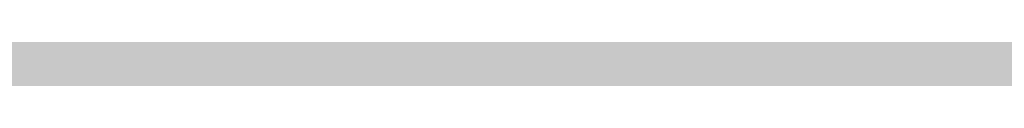
# Model space of a CAD drawing. Units: millimetres. Extents: x 0 to 2267, y 0 to 1823.
# Tile 222 of 256: x 1841.442 to 1842.748, y 1127.423 to 1127.462. Entities that reach past the tile are written whole.
import ezdxf

# ---------------------------------------------------------------- set-up
doc = ezdxf.new("R2010")
doc.units = ezdxf.units.MM
doc.header["$MEASUREMENT"] = 0
doc.layers.add('M-HATC', color=252, linetype='Continuous', lineweight=18)

msp = doc.modelspace()

# ---------------------------------------------------------------- hatches: boundary and pattern name
at = {"layer": 'M-HATC'}
h = msp.add_hatch(color=256, dxfattribs=at)
h.dxf.hatch_style = 1
h.paths.add_polyline_path([(2055.771, 1603.062), (1381.0868, 1603.062), (1381.0868, 1598.062), (2055.771, 1598.062)])
h.paths.add_polyline_path([(2055.771, 1598.062), (1381.0868, 1598.062), (1381.0868, 1593.062), (2055.771, 1593.062)])
h.paths.add_polyline_path([(2051.3074, 1536.7609), (1385.5504, 1536.7609), (1385.5504, 1526.7609), (1387.5504, 1526.7609), (1388.5366, 1525.0528), (1385.3319, 1521.2335), (1385.3319, 1521.2226), (2050.2542, 1522.7491), (2048.3212, 1525.0528), (2049.3074, 1526.7609), (2051.3074, 1526.7609)])
edge = h.paths.add_edge_path()
edge.add_arc((1847.5345, 1379.1492), 135, 222.603061, 222.890851, ccw=False)
edge.add_line((1748.1663, 1287.7656), (1683.0921, 1287.7656))
edge.add_arc((1583.7239, 1379.1492), 135, 317.109149, 317.396939, ccw=False)
edge.add_arc((1678.9686, 1290.6707), 5, 222.8909, 317.1091, ccw=False)
edge.add_arc((1774.2133, 1379.1492), 135, 222.603061, 222.890851, ccw=False)
edge.add_line((1674.8451, 1287.7656), (1609.7709, 1287.7656))
edge.add_arc((1510.4027, 1379.1492), 135, 317.109149, 317.396939, ccw=False)
edge.add_arc((1605.6474, 1290.6707), 5, 222.8909, 317.1091, ccw=False)
edge.add_arc((1700.8921, 1379.1492), 135, 222.603061, 222.890851, ccw=False)
edge.add_line((1601.5239, 1287.7656), (1536.4497, 1287.7656))
edge.add_arc((1437.0815, 1379.1492), 135, 317.109149, 317.396939, ccw=False)
edge.add_arc((1532.3262, 1290.6707), 5, 222.8909, 317.1091, ccw=False)
edge.add_arc((1627.5709, 1379.1492), 135, 222.603061, 222.890851, ccw=False)
edge.add_line((1528.2027, 1287.7656), (1505.9289, 1287.7656))
edge.add_spline(control_points=[(1505.9289, 1287.7656), (1504.2622, 1287.7656), (1504.2622, 1282.7656), (1505.9289, 1282.7656)], knot_values=[0, 0, 0, 0, 5, 5, 5, 5], degree=3, periodic=0)
edge.add_line((1505.9289, 1282.7656), (1930.9289, 1282.7656))
edge.add_spline(control_points=[(1930.9289, 1282.7656), (1932.5956, 1282.7656), (1932.5956, 1287.7656), (1930.9289, 1287.7656)], knot_values=[0, 0, 0, 0, 5, 5, 5, 5], degree=3, periodic=0)
edge.add_line((1930.9289, 1287.7656), (1903.0557, 1287.7656))
edge.add_arc((1803.6875, 1379.1492), 135, 317.109149, 317.396939, ccw=False)
edge.add_arc((1898.9322, 1290.6707), 5, 222.8909, 317.1091, ccw=False)
edge.add_arc((1994.1769, 1379.1492), 135, 222.603061, 222.890851, ccw=False)
edge.add_line((1894.8087, 1287.7656), (1829.7345, 1287.7656))
edge.add_arc((1730.3663, 1379.1492), 135, 317.109149, 317.396939, ccw=False)
edge.add_arc((1825.611, 1290.6707), 5, 222.8909, 317.1091, ccw=False)
edge.add_arc((1920.8557, 1379.1492), 135, 222.603061, 222.890851, ccw=False)
edge.add_line((1821.4875, 1287.7656), (1756.4133, 1287.7656))
edge.add_arc((1657.0451, 1379.1492), 135, 317.109149, 317.396939, ccw=False)
edge.add_arc((1752.2898, 1290.6707), 5, 222.8909, 317.1091, ccw=False)
edge = h.paths.add_edge_path()
edge.add_spline(control_points=[(1843.4289, 1227.2475), (1845.0956, 1227.2475), (1845.0956, 1232.2475), (1843.4289, 1232.2475)], knot_values=[0, 0, 0, 0, 5, 5, 5, 5], degree=3, periodic=0)
edge.add_line((1843.4289, 1232.2475), (1593.4289, 1232.2475))
edge.add_spline(control_points=[(1593.4289, 1232.2475), (1591.7622, 1232.2475), (1591.7622, 1227.2475), (1593.4289, 1227.2475)], knot_values=[0, 0, 0, 0, 5, 5, 5, 5], degree=3, periodic=0)
edge.add_line((1593.4289, 1227.2475), (1843.4289, 1227.2475))
h.paths.add_polyline_path([(1905.9289, 1127.4171), (1530.9289, 1127.4171, 0.414214), (1520.9289, 1117.4171), (1530.9289, 1117.4171), (1915.9289, 1117.4171, 0.414214)])
edge = h.paths.add_edge_path()
edge.add_arc((1397.0858, 1498.4078), 12.7299, 90.78215, 190.87871, ccw=False)
edge.add_line((1396.912, 1511.1365), (1428.0097, 1511.3488))
edge.add_line((1428.0097, 1511.3488), (1433.0097, 1511.3488))
edge.add_line((1433.0097, 1511.3488), (1434.439, 1511.3488))
edge.add_arc((1419.474, 1498.0804), 20, 41.561, 74.08211)
edge.add_line((1424.9592, 1517.3135), (1399.9351, 1517.2561))
edge.add_spline(control_points=[(1399.9307, 1517.2561), (1399.884, 1517.2131), (1399.8328, 1517.1689), (1399.7774, 1517.1236)], knot_values=[11.567499, 11.567499, 11.567499, 11.567499, 11.814249, 11.814249, 11.814249, 11.814249], degree=3, periodic=0)
edge.add_spline(control_points=[(1399.6328, 1517.0099), (1399.5831, 1516.9721), (1399.5307, 1516.9338), (1399.4759, 1516.8947)], knot_values=[11.167718, 11.167718, 11.167718, 11.167718, 11.365188, 11.365188, 11.365188, 11.365188], degree=3, periodic=0)
edge.add_spline(control_points=[(1399.3398, 1516.8001), (1399.1514, 1516.6719), (1398.9384, 1516.5377), (1398.704, 1516.3994)], knot_values=[10.376405, 10.376405, 10.376405, 10.376405, 11.00994, 11.00994, 11.00994, 11.00994], degree=3, periodic=0)
edge.add_spline(control_points=[(1398.6572, 1516.3719), (1398.5789, 1516.326), (1398.4983, 1516.2797), (1398.4155, 1516.2331)], knot_values=[10.125175, 10.125175, 10.125175, 10.125175, 10.334406, 10.334406, 10.334406, 10.334406], degree=3, periodic=0)
edge.add_spline(control_points=[(1398.2642, 1516.1487), (1398.196, 1516.1111), (1398.1263, 1516.0732), (1398.0555, 1516.0351)], knot_values=[9.832246, 9.832246, 9.832246, 9.832246, 9.999658, 9.999658, 9.999658, 9.999658], degree=3, periodic=0)
edge.add_spline(control_points=[(1397.9987, 1516.0048), (1397.7312, 1515.8621), (1397.446, 1515.7171), (1397.1466, 1515.5714)], knot_values=[9.161808, 9.161808, 9.161808, 9.161808, 9.787769, 9.787769, 9.787769, 9.787769], degree=3, periodic=0)
edge.add_spline(control_points=[(1397.1466, 1515.5714), (1396.8418, 1515.423), (1396.5222, 1515.274), (1396.1914, 1515.1262)], knot_values=[8.524455, 8.524455, 8.524455, 8.524455, 9.161808, 9.161808, 9.161808, 9.161808], degree=3, periodic=0)
edge.add_spline(control_points=[(1396.0777, 1515.0756), (1395.9854, 1515.0348), (1395.8922, 1514.994), (1395.7983, 1514.9534)], knot_values=[8.275193, 8.275193, 8.275193, 8.275193, 8.451726, 8.451726, 8.451726, 8.451726], degree=3, periodic=0)
edge.add_spline(control_points=[(1395.6018, 1514.8691), (1395.4997, 1514.8257), (1395.3968, 1514.7824), (1395.2932, 1514.7394)], knot_values=[7.962917, 7.962917, 7.962917, 7.962917, 8.152764, 8.152764, 8.152764, 8.152764], degree=3, periodic=0)
edge.add_spline(control_points=[(1395.2116, 1514.7057), (1394.8278, 1514.5475), (1394.4345, 1514.3929), (1394.0364, 1514.2442)], knot_values=[7.21254, 7.21254, 7.21254, 7.21254, 7.913148, 7.913148, 7.913148, 7.913148], degree=3, periodic=0)
edge.add_spline(control_points=[(1394.0364, 1514.2442), (1393.7076, 1514.1214), (1393.3754, 1514.0027), (1393.0427, 1513.8895)], knot_values=[6.633733, 6.633733, 6.633733, 6.633733, 7.21254, 7.21254, 7.21254, 7.21254], degree=3, periodic=0)
edge.add_spline(control_points=[(1392.8214, 1513.815), (1392.7198, 1513.7812), (1392.6181, 1513.7479), (1392.5166, 1513.7152)], knot_values=[6.328796, 6.328796, 6.328796, 6.328796, 6.505493, 6.505493, 6.505493, 6.505493], degree=3, periodic=0)
edge.add_spline(control_points=[(1392.5166, 1513.7152), (1392.3187, 1513.6515), (1392.1212, 1513.59), (1391.9244, 1513.531)], knot_values=[5.984605, 5.984605, 5.984605, 5.984605, 6.328796, 6.328796, 6.328796, 6.328796], degree=3, periodic=0)
edge.add_spline(control_points=[(1391.7915, 1513.4915), (1391.3122, 1513.3501), (1390.8384, 1513.2239), (1390.3784, 1513.1171)], knot_values=[5.066697, 5.066697, 5.066697, 5.066697, 5.907055, 5.907055, 5.907055, 5.907055], degree=3, periodic=0)
edge.add_spline(control_points=[(1390.3784, 1513.1171), (1390.1797, 1513.071), (1389.9836, 1513.0284), (1389.7907, 1512.9899)], knot_values=[4.70367, 4.70367, 4.70367, 4.70367, 5.066695, 5.066695, 5.066695, 5.066695], degree=3, periodic=0)
edge.add_spline(control_points=[(1389.422, 1512.9204), (1389.2459, 1512.8892), (1389.0729, 1512.8617), (1388.9036, 1512.8381)], knot_values=[4.130571, 4.130571, 4.130571, 4.130571, 4.469816, 4.469816, 4.469816, 4.469816], degree=3, periodic=0)
edge.add_spline(control_points=[(1388.9036, 1512.8381), (1388.591, 1512.7946), (1388.2911, 1512.7644), (1388.0071, 1512.7494)], knot_values=[3.504031, 3.504031, 3.504031, 3.504031, 4.130571, 4.130571, 4.130571, 4.130571], degree=3, periodic=0)
edge.add_spline(control_points=[(1387.9356, 1512.7459), (1387.8538, 1512.7423), (1387.7733, 1512.74), (1387.6944, 1512.739)], knot_values=[3.268866, 3.268866, 3.268866, 3.268866, 3.451164, 3.451164, 3.451164, 3.451164], degree=3, periodic=0)
edge.add_spline(control_points=[(1387.3351, 1512.7443), (1387.2076, 1512.7499), (1387.0847, 1512.7597), (1386.967, 1512.7739)], knot_values=[2.670686, 2.670686, 2.670686, 2.670686, 2.984, 2.984, 2.984, 2.984], degree=3, periodic=0)
edge.add_spline(control_points=[(1386.8327, 1512.7922), (1386.8209, 1512.7941), (1386.8092, 1512.7959), (1386.7975, 1512.7979)], knot_values=[2.516981, 2.516981, 2.516981, 2.516981, 2.549528, 2.549528, 2.549528, 2.549528], degree=3, periodic=0)
edge.add_spline(control_points=[(1386.4526, 1512.8735), (1386.4257, 1512.881), (1386.3993, 1512.889), (1386.3733, 1512.8972)], knot_values=[2.095869, 2.095869, 2.095869, 2.095869, 2.17941, 2.17941, 2.17941, 2.17941], degree=3, periodic=0)
edge.add_spline(control_points=[(1386.0691, 1513.0189), (1386.0634, 1513.0217), (1386.0577, 1513.0246), (1386.052, 1513.0275)], knot_values=[1.72453, 1.72453, 1.72453, 1.72453, 1.745933, 1.745933, 1.745933, 1.745933], degree=3, periodic=0)
edge.add_arc((1399.474, 1498.0804), 20, 131.82432, 180)
edge.add_arc((1630.3336, 1505.5484), 250.9708, 181.705176, 236.427975)
edge.add_arc((1605.3399, 1483.3044), 218.7822, 238.660829, 243.34961)
edge.add_arc((1647.0911, 1510.3592), 262.8986, 183.129836, 237.853442, ccw=False)
h.paths.add_polyline_path([(1406.5369, 1391.9644, 0.149382), (1491.5506, 1296.4418, -0.129517)], flags=17)
edge = h.paths.add_edge_path()
edge.add_arc((2037.3838, 1498.0804), 20, 0, 48.26587)
edge.add_spline(control_points=[(2050.6973, 1513.0052), (2050.6512, 1512.9847), (2050.6034, 1512.9655), (2050.5539, 1512.9477)], knot_values=[1.835652, 1.835652, 1.835652, 1.835652, 2.000781, 2.000781, 2.000781, 2.000781], degree=3, periodic=0)
edge.add_spline(control_points=[(2050.4616, 1512.9166), (2050.479, 1512.9221), (2050.4963, 1512.9277), (2050.5133, 1512.9335)], knot_values=[2.045477, 2.045477, 2.045477, 2.045477, 2.101389, 2.101389, 2.101389, 2.101389], degree=3, periodic=0)
edge.add_spline(control_points=[(2050.129, 1512.8342), (2050.1984, 1512.8473), (2050.2657, 1512.8623), (2050.3308, 1512.8792)], knot_values=[2.237629, 2.237629, 2.237629, 2.237629, 2.435841, 2.435841, 2.435841, 2.435841], degree=3, periodic=0)
edge.add_spline(control_points=[(2050.0946, 1512.8278), (2050.1061, 1512.8299), (2050.1176, 1512.832), (2050.129, 1512.8342)], knot_values=[2.435841, 2.435841, 2.435841, 2.435841, 2.468321, 2.468321, 2.468321, 2.468321], degree=3, periodic=0)
edge.add_spline(control_points=[(2049.7843, 1512.7851), (2049.8552, 1512.7922), (2049.9243, 1512.8008), (2049.9917, 1512.8109)], knot_values=[2.563852, 2.563852, 2.563852, 2.563852, 2.748541, 2.748541, 2.748541, 2.748541], degree=3, periodic=0)
edge.add_spline(control_points=[(2049.4052, 1512.7617), (2049.5364, 1512.7653), (2049.6629, 1512.773), (2049.7843, 1512.7851)], knot_values=[2.748541, 2.748541, 2.748541, 2.748541, 3.064882, 3.064882, 3.064882, 3.064882], degree=3, periodic=0)
edge.add_spline(control_points=[(2049.1698, 1512.7597), (2049.2336, 1512.7591), (2049.2965, 1512.7594), (2049.3584, 1512.7606)], knot_values=[3.102309, 3.102309, 3.102309, 3.102309, 3.2503, 3.2503, 3.2503, 3.2503], degree=3, periodic=0)
edge.add_spline(control_points=[(2048.8573, 1512.7691), (2048.9638, 1512.7638), (2049.068, 1512.7606), (2049.1698, 1512.7597)], knot_values=[3.2503, 3.2503, 3.2503, 3.2503, 3.486069, 3.486069, 3.486069, 3.486069], degree=3, periodic=0)
edge.add_spline(control_points=[(2048.6924, 1512.7789), (2048.3729, 1512.8009), (2048.0345, 1512.8411), (2047.6817, 1512.897)], knot_values=[3.606429, 3.606429, 3.606429, 3.606429, 4.2989, 4.2989, 4.2989, 4.2989], degree=3, periodic=0)
edge.add_spline(control_points=[(2047.6817, 1512.897), (2047.5458, 1512.9185), (2047.4077, 1512.9424), (2047.2678, 1512.9685)], knot_values=[4.2989, 4.2989, 4.2989, 4.2989, 4.565769, 4.565769, 4.565769, 4.565769], degree=3, periodic=0)
edge.add_spline(control_points=[(2047.2678, 1512.9685), (2047.1449, 1512.9914), (2047.0207, 1513.016), (2046.8951, 1513.0422)], knot_values=[4.565769, 4.565769, 4.565769, 4.565769, 4.799971, 4.799971, 4.799971, 4.799971], degree=3, periodic=0)
edge.add_spline(control_points=[(2046.8951, 1513.0422), (2046.5286, 1513.1188), (2046.1513, 1513.209), (2045.7676, 1513.3107)], knot_values=[4.799971, 4.799971, 4.799971, 4.799971, 5.483718, 5.483718, 5.483718, 5.483718], degree=3, periodic=0)
edge.add_spline(control_points=[(2045.7676, 1513.3107), (2045.3724, 1513.4154), (2044.9704, 1513.5322), (2044.5662, 1513.6588)], knot_values=[5.483718, 5.483718, 5.483718, 5.483718, 6.187866, 6.187866, 6.187866, 6.187866], degree=3, periodic=0)
edge.add_spline(control_points=[(2044.5662, 1513.6588), (2044.4149, 1513.7061), (2044.2633, 1513.7549), (2044.1116, 1513.8048)], knot_values=[6.187866, 6.187866, 6.187866, 6.187866, 6.451551, 6.451551, 6.451551, 6.451551], degree=3, periodic=0)
edge.add_spline(control_points=[(2044.1116, 1513.8048), (2043.9967, 1513.8427), (2043.8817, 1513.8813), (2043.7668, 1513.9205)], knot_values=[6.451551, 6.451551, 6.451551, 6.451551, 6.651434, 6.651434, 6.651434, 6.651434], degree=3, periodic=0)
edge.add_spline(control_points=[(2043.7668, 1513.9205), (2043.3716, 1514.0554), (2042.9774, 1514.1979), (2042.5886, 1514.3458)], knot_values=[6.651434, 6.651434, 6.651434, 6.651434, 7.338879, 7.338879, 7.338879, 7.338879], degree=3, periodic=0)
edge.add_spline(control_points=[(2042.5886, 1514.3458), (2042.1643, 1514.5071), (2041.7465, 1514.6749), (2041.3409, 1514.846)], knot_values=[7.338879, 7.338879, 7.338879, 7.338879, 8.089209, 8.089209, 8.089209, 8.089209], degree=3, periodic=0)
edge.add_spline(control_points=[(2041.3409, 1514.846), (2041.1028, 1514.9465), (2040.869, 1515.0481), (2040.6405, 1515.1502)], knot_values=[8.089209, 8.089209, 8.089209, 8.089209, 8.529587, 8.529587, 8.529587, 8.529587], degree=3, periodic=0)
edge.add_spline(control_points=[(2040.51, 1515.2089), (2040.0824, 1515.4022), (2039.6747, 1515.5971), (2039.295, 1515.7894)], knot_values=[8.613818, 8.613818, 8.613818, 8.613818, 9.44571, 9.44571, 9.44571, 9.44571], degree=3, periodic=0)
edge.add_spline(control_points=[(2039.295, 1515.7894), (2039.0618, 1515.9075), (2038.8391, 1516.0246), (2038.6288, 1516.1398)], knot_values=[9.44571, 9.44571, 9.44571, 9.44571, 9.956404, 9.956404, 9.956404, 9.956404], degree=3, periodic=0)
edge.add_spline(control_points=[(2038.6288, 1516.1398), (2038.5187, 1516.2001), (2038.4121, 1516.2598), (2038.309, 1516.3189)], knot_values=[9.956404, 9.956404, 9.956404, 9.956404, 10.223542, 10.223542, 10.223542, 10.223542], degree=3, periodic=0)
edge.add_spline(control_points=[(2038.309, 1516.3189), (2038.2138, 1516.3735), (2038.1216, 1516.4276), (2038.0328, 1516.481)], knot_values=[10.223542, 10.223542, 10.223542, 10.223542, 10.47051, 10.47051, 10.47051, 10.47051], degree=3, periodic=0)
edge.add_spline(control_points=[(2038.0328, 1516.481), (2037.7855, 1516.6296), (2037.5639, 1516.773), (2037.3722, 1516.909)], knot_values=[10.47051, 10.47051, 10.47051, 10.47051, 11.15767, 11.15767, 11.15767, 11.15767], degree=3, periodic=0)
edge.add_spline(control_points=[(2037.3722, 1516.909), (2037.2789, 1516.9752), (2037.1927, 1517.0396), (2037.1142, 1517.102)], knot_values=[11.15767, 11.15767, 11.15767, 11.15767, 11.49227, 11.49227, 11.49227, 11.49227], degree=3, periodic=0)
edge.add_spline(control_points=[(2036.8564, 1517.3259), (2036.9148, 1517.2692), (2036.9814, 1517.2103), (2037.0557, 1517.1492)], knot_values=[11.577341, 11.577341, 11.577341, 11.577341, 11.91035, 11.91035, 11.91035, 11.91035], degree=3, periodic=0)
edge.add_spline(control_points=[(2036.8074, 1517.3748), (2036.823, 1517.3587), (2036.8393, 1517.3424), (2036.8564, 1517.3259)], knot_values=[11.91035, 11.91035, 11.91035, 11.91035, 12.007402, 12.007402, 12.007402, 12.007402], degree=3, periodic=0)
edge.add_spline(control_points=[(2036.7017, 1517.494), (2036.7104, 1517.483), (2036.7196, 1517.4719), (2036.7291, 1517.4606)], knot_values=[12.184155, 12.184155, 12.184155, 12.184155, 12.255409, 12.255409, 12.255409, 12.255409], degree=3, periodic=0)
edge.add_spline(control_points=[(2036.6159, 1517.6205), (2036.62, 1517.613), (2036.6243, 1517.6055), (2036.6289, 1517.5979)], knot_values=[12.487913, 12.487913, 12.487913, 12.487913, 12.541035, 12.541035, 12.541035, 12.541035], degree=3, periodic=0)
edge.add_spline(control_points=[(2036.5635, 1517.786), (2036.5637, 1517.7794), (2036.5642, 1517.7726), (2036.565, 1517.7658)], knot_values=[12.911761, 12.911761, 12.911761, 12.911761, 12.968286, 12.968286, 12.968286, 12.968286], degree=3, periodic=0)
edge.add_spline(control_points=[(2036.6166, 1517.9304), (2036.6125, 1517.9259), (2036.6086, 1517.9212), (2036.6049, 1517.9165)], knot_values=[13.382527, 13.382527, 13.382527, 13.382527, 13.433791, 13.433791, 13.433791, 13.433791], degree=3, periodic=0)
edge.add_spline(control_points=[(2036.749, 1518.017), (2036.7361, 1518.0116), (2036.7239, 1518.006), (2036.7124, 1518.0002)], knot_values=[13.726299, 13.726299, 13.726299, 13.726299, 13.809928, 13.809928, 13.809928, 13.809928], degree=3, periodic=0)
edge.add_spline(control_points=[(2036.8604, 1518.0528), (2036.8386, 1518.0474), (2036.8181, 1518.0416), (2036.7988, 1518.0353)], knot_values=[13.910887, 13.910887, 13.910887, 13.910887, 14.02153, 14.02153, 14.02153, 14.02153], degree=3, periodic=0)
edge.add_line((2036.9639, 1518.0804), (2032.3838, 1518.0804))
edge.add_line((2032.3838, 1518.0804), (2027.3838, 1518.0804))
edge.add_line((2027.3838, 1518.0804), (2022.3838, 1518.0804))
edge.add_line((2022.3838, 1518.0804), (2017.3838, 1518.0804))
edge.add_arc((2017.3838, 1498.0804), 20, 90, 138.439)
edge.add_line((2002.4188, 1511.3488), (2003.8481, 1511.3488))
edge.add_line((2003.8481, 1511.3488), (2008.8481, 1511.3488))
edge.add_line((2008.8481, 1511.3488), (2039.772, 1511.1377))
edge.add_arc((2039.772, 1498.4078), 12.7299, -10.87871, 90, ccw=False)
edge.add_arc((1789.7668, 1510.3592), 262.8986, 302.146558, 356.870164, ccw=False)
edge.add_arc((1831.5179, 1483.3044), 218.7822, 296.65039, 301.339171)
edge.add_arc((1806.5242, 1505.5484), 250.9708, 303.572025, 358.294824)
h.paths.add_polyline_path([(2030.321, 1391.9644, -0.129517), (1945.3072, 1296.4418, 0.149382)], flags=17)
edge = h.paths.add_edge_path()
edge.add_spline(control_points=[(2037.2464, 1518.0821), (2037.2898, 1518.081), (2037.3355, 1518.0804), (2037.3838, 1518.0804)], knot_values=[0.000012, 0.000012, 0.000012, 0.000012, 0.144754, 0.144754, 0.144754, 0.144754], degree=3, periodic=0)
edge.add_line((2037.3357, 1518.0804), (2037.0096, 1518.0804))
edge.add_spline(control_points=[(2037.0096, 1518.0804), (2036.9822, 1518.0768), (2036.956, 1518.0727), (2036.9312, 1518.0681)], knot_values=[14.13465, 14.13465, 14.13465, 14.13465, 14.247197, 14.247197, 14.247197, 14.247197], degree=3, periodic=0)
edge.add_spline(control_points=[(2036.9312, 1518.0681), (2036.9276, 1518.0674), (2036.9241, 1518.0667), (2036.9205, 1518.0661)], knot_values=[14.118315, 14.118315, 14.118315, 14.118315, 14.13465, 14.13465, 14.13465, 14.13465], degree=3, periodic=0)
edge.add_spline(control_points=[(2036.9205, 1518.0661), (2036.9118, 1518.0644), (2036.9032, 1518.0626), (2036.8948, 1518.0608)], knot_values=[14.078086, 14.078086, 14.078086, 14.078086, 14.118315, 14.118315, 14.118315, 14.118315], degree=3, periodic=0)
edge.add_spline(control_points=[(2036.8948, 1518.0608), (2036.883, 1518.0583), (2036.8716, 1518.0556), (2036.8604, 1518.0528)], knot_values=[14.02153, 14.02153, 14.02153, 14.02153, 14.078086, 14.078086, 14.078086, 14.078086], degree=3, periodic=0)
edge.add_spline(control_points=[(2036.8604, 1518.0528), (2036.8386, 1518.0474), (2036.8181, 1518.0416), (2036.7988, 1518.0353)], knot_values=[13.910887, 13.910887, 13.910887, 13.910887, 14.02153, 14.02153, 14.02153, 14.02153], degree=3, periodic=0)
edge.add_spline(control_points=[(2036.7988, 1518.0353), (2036.7981, 1518.035), (2036.7974, 1518.0348), (2036.7967, 1518.0346)], knot_values=[13.906906, 13.906906, 13.906906, 13.906906, 13.910887, 13.910887, 13.910887, 13.910887], degree=3, periodic=0)
edge.add_spline(control_points=[(2036.7967, 1518.0346), (2036.7882, 1518.0318), (2036.7799, 1518.0289), (2036.7719, 1518.0259)], knot_values=[13.857826, 13.857826, 13.857826, 13.857826, 13.906906, 13.906906, 13.906906, 13.906906], degree=3, periodic=0)
edge.add_spline(control_points=[(2036.7719, 1518.0259), (2036.764, 1518.023), (2036.7564, 1518.02), (2036.749, 1518.017)], knot_values=[13.809928, 13.809928, 13.809928, 13.809928, 13.857826, 13.857826, 13.857826, 13.857826], degree=3, periodic=0)
edge.add_spline(control_points=[(2036.749, 1518.017), (2036.7361, 1518.0116), (2036.7239, 1518.006), (2036.7124, 1518.0002)], knot_values=[13.726299, 13.726299, 13.726299, 13.726299, 13.809928, 13.809928, 13.809928, 13.809928], degree=3, periodic=0)
edge.add_spline(control_points=[(2036.7124, 1518.0002), (2036.7121, 1518), (2036.7118, 1517.9999), (2036.7115, 1517.9997)], knot_values=[13.723993, 13.723993, 13.723993, 13.723993, 13.726299, 13.726299, 13.726299, 13.726299], degree=3, periodic=0)
edge.add_spline(control_points=[(2036.7115, 1517.9997), (2036.7063, 1517.9971), (2036.7013, 1517.9944), (2036.6965, 1517.9917)], knot_values=[13.686536, 13.686536, 13.686536, 13.686536, 13.723993, 13.723993, 13.723993, 13.723993], degree=3, periodic=0)
edge.add_spline(control_points=[(2036.6965, 1517.9917), (2036.6919, 1517.9891), (2036.6874, 1517.9865), (2036.6831, 1517.9839)], knot_values=[13.651251, 13.651251, 13.651251, 13.651251, 13.686536, 13.686536, 13.686536, 13.686536], degree=3, periodic=0)
edge.add_spline(control_points=[(2036.6831, 1517.9839), (2036.6764, 1517.9798), (2036.67, 1517.9757), (2036.6639, 1517.9714)], knot_values=[13.596804, 13.596804, 13.596804, 13.596804, 13.651251, 13.651251, 13.651251, 13.651251], degree=3, periodic=0)
edge.add_spline(control_points=[(2036.6639, 1517.9714), (2036.6636, 1517.9712), (2036.6633, 1517.9709), (2036.6629, 1517.9707)], knot_values=[13.593956, 13.593956, 13.593956, 13.593956, 13.596804, 13.596804, 13.596804, 13.596804], degree=3, periodic=0)
edge.add_spline(control_points=[(2036.6629, 1517.9707), (2036.6603, 1517.9689), (2036.6577, 1517.967), (2036.6552, 1517.9651)], knot_values=[13.570322, 13.570322, 13.570322, 13.570322, 13.593956, 13.593956, 13.593956, 13.593956], degree=3, periodic=0)
edge.add_spline(control_points=[(2036.6552, 1517.9651), (2036.6525, 1517.9631), (2036.6499, 1517.9611), (2036.6474, 1517.9591)], knot_values=[13.545477, 13.545477, 13.545477, 13.545477, 13.570322, 13.570322, 13.570322, 13.570322], degree=3, periodic=0)
edge.add_spline(control_points=[(2036.6474, 1517.9591), (2036.6472, 1517.9589), (2036.6471, 1517.9588), (2036.6469, 1517.9587)], knot_values=[13.543931, 13.543931, 13.543931, 13.543931, 13.545477, 13.545477, 13.545477, 13.545477], degree=3, periodic=0)
edge.add_spline(control_points=[(2036.6469, 1517.9587), (2036.6412, 1517.9541), (2036.6358, 1517.9494), (2036.6307, 1517.9447)], knot_values=[13.488237, 13.488237, 13.488237, 13.488237, 13.543931, 13.543931, 13.543931, 13.543931], degree=3, periodic=0)
edge.add_spline(control_points=[(2036.6307, 1517.9447), (2036.6282, 1517.9423), (2036.6257, 1517.9399), (2036.6233, 1517.9374)], knot_values=[13.460307, 13.460307, 13.460307, 13.460307, 13.488237, 13.488237, 13.488237, 13.488237], degree=3, periodic=0)
edge.add_spline(control_points=[(2036.6233, 1517.9374), (2036.6215, 1517.9356), (2036.6198, 1517.9338), (2036.6181, 1517.932)], knot_values=[13.439712, 13.439712, 13.439712, 13.439712, 13.460307, 13.460307, 13.460307, 13.460307], degree=3, periodic=0)
edge.add_spline(control_points=[(2036.6181, 1517.932), (2036.6176, 1517.9315), (2036.6171, 1517.9309), (2036.6166, 1517.9304)], knot_values=[13.433791, 13.433791, 13.433791, 13.433791, 13.439712, 13.439712, 13.439712, 13.439712], degree=3, periodic=0)
edge.add_spline(control_points=[(2036.6166, 1517.9304), (2036.6125, 1517.9259), (2036.6086, 1517.9212), (2036.6049, 1517.9165)], knot_values=[13.382527, 13.382527, 13.382527, 13.382527, 13.433791, 13.433791, 13.433791, 13.433791], degree=3, periodic=0)
edge.add_spline(control_points=[(2036.6049, 1517.9165), (2036.6026, 1517.9135), (2036.6004, 1517.9104), (2036.5982, 1517.9074)], knot_values=[13.350017, 13.350017, 13.350017, 13.350017, 13.382527, 13.382527, 13.382527, 13.382527], degree=3, periodic=0)
edge.add_spline(control_points=[(2036.5982, 1517.9074), (2036.5972, 1517.9059), (2036.5962, 1517.9043), (2036.5952, 1517.9028)], knot_values=[13.333922, 13.333922, 13.333922, 13.333922, 13.350017, 13.350017, 13.350017, 13.350017], degree=3, periodic=0)
edge.add_spline(control_points=[(2036.5952, 1517.9028), (2036.5945, 1517.9018), (2036.5939, 1517.9009), (2036.5933, 1517.8999)], knot_values=[13.323828, 13.323828, 13.323828, 13.323828, 13.333922, 13.333922, 13.333922, 13.333922], degree=3, periodic=0)
edge.add_spline(control_points=[(2036.5933, 1517.8999), (2036.5905, 1517.8955), (2036.5879, 1517.8909), (2036.5855, 1517.8864)], knot_values=[13.277545, 13.277545, 13.277545, 13.277545, 13.323828, 13.323828, 13.323828, 13.323828], degree=3, periodic=0)
edge.add_spline(control_points=[(2036.5855, 1517.8864), (2036.5836, 1517.8827), (2036.5817, 1517.8789), (2036.5801, 1517.8751)], knot_values=[13.240119, 13.240119, 13.240119, 13.240119, 13.277545, 13.277545, 13.277545, 13.277545], degree=3, periodic=0)
edge.add_spline(control_points=[(2036.5801, 1517.8751), (2036.5795, 1517.8739), (2036.579, 1517.8727), (2036.5785, 1517.8715)], knot_values=[13.228211, 13.228211, 13.228211, 13.228211, 13.240119, 13.240119, 13.240119, 13.240119], degree=3, periodic=0)
edge.add_spline(control_points=[(2036.5785, 1517.8715), (2036.578, 1517.8702), (2036.5774, 1517.869), (2036.5769, 1517.8677)], knot_values=[13.215717, 13.215717, 13.215717, 13.215717, 13.228211, 13.228211, 13.228211, 13.228211], degree=3, periodic=0)
edge.add_spline(control_points=[(2036.5769, 1517.8677), (2036.5755, 1517.864), (2036.5741, 1517.8603), (2036.5729, 1517.8565)], knot_values=[13.179847, 13.179847, 13.179847, 13.179847, 13.215717, 13.215717, 13.215717, 13.215717], degree=3, periodic=0)
edge.add_spline(control_points=[(2036.5729, 1517.8565), (2036.5713, 1517.8515), (2036.5699, 1517.8464), (2036.5687, 1517.8413)], knot_values=[13.132017, 13.132017, 13.132017, 13.132017, 13.179847, 13.179847, 13.179847, 13.179847], degree=3, periodic=0)
edge.add_spline(control_points=[(2036.5687, 1517.8413), (2036.5684, 1517.8402), (2036.5682, 1517.8392), (2036.568, 1517.8382)], knot_values=[13.122482, 13.122482, 13.122482, 13.122482, 13.132017, 13.132017, 13.132017, 13.132017], degree=3, periodic=0)
edge.add_spline(control_points=[(2036.568, 1517.8382), (2036.5676, 1517.8363), (2036.5672, 1517.8345), (2036.5669, 1517.8327)], knot_values=[13.105592, 13.105592, 13.105592, 13.105592, 13.122482, 13.122482, 13.122482, 13.122482], degree=3, periodic=0)
edge.add_spline(control_points=[(2036.5669, 1517.8327), (2036.5662, 1517.8292), (2036.5657, 1517.8257), (2036.5652, 1517.8222)], knot_values=[13.074063, 13.074063, 13.074063, 13.074063, 13.105592, 13.105592, 13.105592, 13.105592], degree=3, periodic=0)
edge.add_spline(control_points=[(2036.5652, 1517.8222), (2036.5652, 1517.8222), (2036.5652, 1517.8222), (2036.5652, 1517.8222)], knot_values=[13.074043, 13.074043, 13.074043, 13.074043, 13.074063, 13.074063, 13.074063, 13.074063], degree=3, periodic=0)
edge.add_spline(control_points=[(2036.5652, 1517.8222), (2036.5644, 1517.8164), (2036.5639, 1517.8106), (2036.5636, 1517.8046)], knot_values=[13.021884, 13.021884, 13.021884, 13.021884, 13.074043, 13.074043, 13.074043, 13.074043], degree=3, periodic=0)
edge.add_spline(control_points=[(2036.5636, 1517.8046), (2036.5636, 1517.804), (2036.5636, 1517.8034), (2036.5635, 1517.8028)], knot_values=[13.01674, 13.01674, 13.01674, 13.01674, 13.021884, 13.021884, 13.021884, 13.021884], degree=3, periodic=0)
edge.add_spline(control_points=[(2036.5635, 1517.8028), (2036.5634, 1517.8005), (2036.5634, 1517.7982), (2036.5634, 1517.7958)], knot_values=[12.996438, 12.996438, 12.996438, 12.996438, 13.01674, 13.01674, 13.01674, 13.01674], degree=3, periodic=0)
edge.add_spline(control_points=[(2036.5634, 1517.7958), (2036.5633, 1517.7926), (2036.5634, 1517.7893), (2036.5635, 1517.786)], knot_values=[12.968286, 12.968286, 12.968286, 12.968286, 12.996438, 12.996438, 12.996438, 12.996438], degree=3, periodic=0)
edge.add_spline(control_points=[(2036.5635, 1517.786), (2036.5637, 1517.7794), (2036.5642, 1517.7726), (2036.565, 1517.7658)], knot_values=[12.911761, 12.911761, 12.911761, 12.911761, 12.968286, 12.968286, 12.968286, 12.968286], degree=3, periodic=0)
edge.add_spline(control_points=[(2036.565, 1517.7658), (2036.565, 1517.7657), (2036.565, 1517.7656), (2036.565, 1517.7656)], knot_values=[12.911017, 12.911017, 12.911017, 12.911017, 12.911761, 12.911761, 12.911761, 12.911761], degree=3, periodic=0)
edge.add_spline(control_points=[(2036.565, 1517.7656), (2036.5654, 1517.7625), (2036.5658, 1517.7593), (2036.5663, 1517.7562)], knot_values=[12.88528, 12.88528, 12.88528, 12.88528, 12.911017, 12.911017, 12.911017, 12.911017], degree=3, periodic=0)
edge.add_spline(control_points=[(2036.5663, 1517.7562), (2036.5667, 1517.7534), (2036.5672, 1517.7506), (2036.5677, 1517.7478)], knot_values=[12.862519, 12.862519, 12.862519, 12.862519, 12.88528, 12.88528, 12.88528, 12.88528], degree=3, periodic=0)
edge.add_spline(control_points=[(2036.5677, 1517.7478), (2036.5678, 1517.7474), (2036.5679, 1517.7469), (2036.568, 1517.7465)], knot_values=[12.858885, 12.858885, 12.858885, 12.858885, 12.862519, 12.862519, 12.862519, 12.862519], degree=3, periodic=0)
edge.add_spline(control_points=[(2036.568, 1517.7465), (2036.5692, 1517.7399), (2036.5707, 1517.7332), (2036.5724, 1517.7264)], knot_values=[12.8053, 12.8053, 12.8053, 12.8053, 12.858885, 12.858885, 12.858885, 12.858885], degree=3, periodic=0)
edge.add_spline(control_points=[(2036.5724, 1517.7264), (2036.5734, 1517.7226), (2036.5745, 1517.7187), (2036.5756, 1517.7149)], knot_values=[12.775176, 12.775176, 12.775176, 12.775176, 12.8053, 12.8053, 12.8053, 12.8053], degree=3, periodic=0)
edge.add_spline(control_points=[(2036.5756, 1517.7149), (2036.5763, 1517.7125), (2036.577, 1517.7102), (2036.5778, 1517.7078)], knot_values=[12.756759, 12.756759, 12.756759, 12.756759, 12.775176, 12.775176, 12.775176, 12.775176], degree=3, periodic=0)
edge.add_spline(control_points=[(2036.5778, 1517.7078), (2036.5781, 1517.7067), (2036.5784, 1517.7057), (2036.5787, 1517.7047)], knot_values=[12.748742, 12.748742, 12.748742, 12.748742, 12.756759, 12.756759, 12.756759, 12.756759], degree=3, periodic=0)
edge.add_spline(control_points=[(2036.5787, 1517.7047), (2036.5808, 1517.6983), (2036.5831, 1517.6919), (2036.5856, 1517.6854)], knot_values=[12.69959, 12.69959, 12.69959, 12.69959, 12.748742, 12.748742, 12.748742, 12.748742], degree=3, periodic=0)
edge.add_spline(control_points=[(2036.5856, 1517.6854), (2036.5876, 1517.68), (2036.5898, 1517.6746), (2036.5921, 1517.6692)], knot_values=[12.659038, 12.659038, 12.659038, 12.659038, 12.69959, 12.69959, 12.69959, 12.69959], degree=3, periodic=0)
edge.add_spline(control_points=[(2036.5921, 1517.6692), (2036.594, 1517.6648), (2036.5959, 1517.6605), (2036.5979, 1517.6561)], knot_values=[12.626806, 12.626806, 12.626806, 12.626806, 12.659038, 12.659038, 12.659038, 12.659038], degree=3, periodic=0)
edge.add_spline(control_points=[(2036.5979, 1517.6561), (2036.5984, 1517.6551), (2036.5989, 1517.6541), (2036.5993, 1517.6531)], knot_values=[12.619394, 12.619394, 12.619394, 12.619394, 12.626806, 12.626806, 12.626806, 12.626806], degree=3, periodic=0)
edge.add_spline(control_points=[(2036.5993, 1517.6531), (2036.6043, 1517.6424), (2036.6099, 1517.6315), (2036.6159, 1517.6205)], knot_values=[12.541039, 12.541039, 12.541039, 12.541039, 12.619394, 12.619394, 12.619394, 12.619394], degree=3, periodic=0)
edge.add_spline(control_points=[(2036.6159, 1517.6205), (2036.6159, 1517.6205), (2036.6159, 1517.6205), (2036.6159, 1517.6205)], knot_values=[12.541035, 12.541035, 12.541035, 12.541035, 12.541039, 12.541039, 12.541039, 12.541039], degree=3, periodic=0)
edge.add_spline(control_points=[(2036.6159, 1517.6205), (2036.62, 1517.613), (2036.6243, 1517.6055), (2036.6289, 1517.5979)], knot_values=[12.487913, 12.487913, 12.487913, 12.487913, 12.541035, 12.541035, 12.541035, 12.541035], degree=3, periodic=0)
edge.add_spline(control_points=[(2036.6289, 1517.5979), (2036.6326, 1517.5916), (2036.6365, 1517.5853), (2036.6406, 1517.5789)], knot_values=[12.443982, 12.443982, 12.443982, 12.443982, 12.487913, 12.487913, 12.487913, 12.487913], degree=3, periodic=0)
edge.add_spline(control_points=[(2036.6406, 1517.5789), (2036.6414, 1517.5776), (2036.6423, 1517.5763), (2036.6431, 1517.5749)], knot_values=[12.434996, 12.434996, 12.434996, 12.434996, 12.443982, 12.443982, 12.443982, 12.443982], degree=3, periodic=0)
edge.add_spline(control_points=[(2036.6431, 1517.5749), (2036.6531, 1517.5596), (2036.6639, 1517.5439), (2036.6756, 1517.528)], knot_values=[12.329647, 12.329647, 12.329647, 12.329647, 12.434996, 12.434996, 12.434996, 12.434996], degree=3, periodic=0)
edge.add_spline(control_points=[(2036.6756, 1517.528), (2036.6839, 1517.5168), (2036.6925, 1517.5055), (2036.7017, 1517.494)], knot_values=[12.255409, 12.255409, 12.255409, 12.255409, 12.329647, 12.329647, 12.329647, 12.329647], degree=3, periodic=0)
edge.add_spline(control_points=[(2036.7017, 1517.494), (2036.7104, 1517.483), (2036.7196, 1517.4719), (2036.7291, 1517.4606)], knot_values=[12.184155, 12.184155, 12.184155, 12.184155, 12.255409, 12.255409, 12.255409, 12.255409], degree=3, periodic=0)
edge.add_spline(control_points=[(2036.7291, 1517.4606), (2036.7436, 1517.4435), (2036.759, 1517.4262), (2036.7753, 1517.4085)], knot_values=[12.075961, 12.075961, 12.075961, 12.075961, 12.184155, 12.184155, 12.184155, 12.184155], degree=3, periodic=0)
edge.add_spline(control_points=[(2036.7753, 1517.4085), (2036.7763, 1517.4075), (2036.7773, 1517.4064), (2036.7783, 1517.4054)], knot_values=[12.069502, 12.069502, 12.069502, 12.069502, 12.075961, 12.075961, 12.075961, 12.075961], degree=3, periodic=0)
edge.add_spline(control_points=[(2036.7783, 1517.4054), (2036.7877, 1517.3953), (2036.7974, 1517.385), (2036.8074, 1517.3748)], knot_values=[12.007402, 12.007402, 12.007402, 12.007402, 12.069502, 12.069502, 12.069502, 12.069502], degree=3, periodic=0)
edge.add_spline(control_points=[(2036.8074, 1517.3748), (2036.823, 1517.3587), (2036.8393, 1517.3424), (2036.8564, 1517.3259)], knot_values=[11.91035, 11.91035, 11.91035, 11.91035, 12.007402, 12.007402, 12.007402, 12.007402], degree=3, periodic=0)
edge.add_spline(control_points=[(2036.8564, 1517.3259), (2036.9148, 1517.2692), (2036.9814, 1517.2103), (2037.0557, 1517.1492)], knot_values=[11.577341, 11.577341, 11.577341, 11.577341, 11.91035, 11.91035, 11.91035, 11.91035], degree=3, periodic=0)
edge.add_spline(control_points=[(2037.0557, 1517.1492), (2037.0747, 1517.1336), (2037.0942, 1517.1179), (2037.1142, 1517.102)], knot_values=[11.49227, 11.49227, 11.49227, 11.49227, 11.577341, 11.577341, 11.577341, 11.577341], degree=3, periodic=0)
edge.add_spline(control_points=[(2037.1142, 1517.102), (2037.1927, 1517.0396), (2037.2789, 1516.9752), (2037.3722, 1516.909)], knot_values=[11.15767, 11.15767, 11.15767, 11.15767, 11.49227, 11.49227, 11.49227, 11.49227], degree=3, periodic=0)
edge.add_spline(control_points=[(2037.3722, 1516.909), (2037.5639, 1516.773), (2037.7855, 1516.6296), (2038.0328, 1516.481)], knot_values=[10.47051, 10.47051, 10.47051, 10.47051, 11.15767, 11.15767, 11.15767, 11.15767], degree=3, periodic=0)
edge.add_spline(control_points=[(2038.0328, 1516.481), (2038.1216, 1516.4276), (2038.2138, 1516.3735), (2038.309, 1516.3189)], knot_values=[10.223542, 10.223542, 10.223542, 10.223542, 10.47051, 10.47051, 10.47051, 10.47051], degree=3, periodic=0)
edge.add_spline(control_points=[(2038.309, 1516.3189), (2038.4121, 1516.2598), (2038.5187, 1516.2001), (2038.6288, 1516.1398)], knot_values=[9.956404, 9.956404, 9.956404, 9.956404, 10.223542, 10.223542, 10.223542, 10.223542], degree=3, periodic=0)
edge.add_spline(control_points=[(2038.6288, 1516.1398), (2038.8391, 1516.0246), (2039.0618, 1515.9075), (2039.295, 1515.7894)], knot_values=[9.44571, 9.44571, 9.44571, 9.44571, 9.956404, 9.956404, 9.956404, 9.956404], degree=3, periodic=0)
edge.add_spline(control_points=[(2039.295, 1515.7894), (2039.6747, 1515.5971), (2040.0824, 1515.4022), (2040.51, 1515.2089)], knot_values=[8.613818, 8.613818, 8.613818, 8.613818, 9.44571, 9.44571, 9.44571, 9.44571], degree=3, periodic=0)
edge.add_spline(control_points=[(2040.51, 1515.2089), (2040.5533, 1515.1893), (2040.5968, 1515.1697), (2040.6405, 1515.1502)], knot_values=[8.529587, 8.529587, 8.529587, 8.529587, 8.613818, 8.613818, 8.613818, 8.613818], degree=3, periodic=0)
edge.add_spline(control_points=[(2040.6405, 1515.1502), (2040.869, 1515.0481), (2041.1028, 1514.9465), (2041.3409, 1514.846)], knot_values=[8.089209, 8.089209, 8.089209, 8.089209, 8.529587, 8.529587, 8.529587, 8.529587], degree=3, periodic=0)
edge.add_spline(control_points=[(2041.3409, 1514.846), (2041.7465, 1514.6749), (2042.1643, 1514.5071), (2042.5886, 1514.3458)], knot_values=[7.338879, 7.338879, 7.338879, 7.338879, 8.089209, 8.089209, 8.089209, 8.089209], degree=3, periodic=0)
edge.add_spline(control_points=[(2042.5886, 1514.3458), (2042.9774, 1514.1979), (2043.3716, 1514.0554), (2043.7668, 1513.9205)], knot_values=[6.651434, 6.651434, 6.651434, 6.651434, 7.338879, 7.338879, 7.338879, 7.338879], degree=3, periodic=0)
edge.add_spline(control_points=[(2043.7668, 1513.9205), (2043.8817, 1513.8813), (2043.9967, 1513.8427), (2044.1116, 1513.8048)], knot_values=[6.451551, 6.451551, 6.451551, 6.451551, 6.651434, 6.651434, 6.651434, 6.651434], degree=3, periodic=0)
edge.add_spline(control_points=[(2044.1116, 1513.8048), (2044.2633, 1513.7549), (2044.4149, 1513.7061), (2044.5662, 1513.6588)], knot_values=[6.187866, 6.187866, 6.187866, 6.187866, 6.451551, 6.451551, 6.451551, 6.451551], degree=3, periodic=0)
edge.add_spline(control_points=[(2044.5662, 1513.6588), (2044.9704, 1513.5322), (2045.3724, 1513.4154), (2045.7676, 1513.3107)], knot_values=[5.483718, 5.483718, 5.483718, 5.483718, 6.187866, 6.187866, 6.187866, 6.187866], degree=3, periodic=0)
edge.add_spline(control_points=[(2045.7676, 1513.3107), (2046.1513, 1513.209), (2046.5286, 1513.1188), (2046.8951, 1513.0422)], knot_values=[4.799971, 4.799971, 4.799971, 4.799971, 5.483718, 5.483718, 5.483718, 5.483718], degree=3, periodic=0)
edge.add_spline(control_points=[(2046.8951, 1513.0422), (2047.0207, 1513.016), (2047.1449, 1512.9914), (2047.2678, 1512.9685)], knot_values=[4.565769, 4.565769, 4.565769, 4.565769, 4.799971, 4.799971, 4.799971, 4.799971], degree=3, periodic=0)
edge.add_spline(control_points=[(2047.2678, 1512.9685), (2047.4077, 1512.9424), (2047.5458, 1512.9185), (2047.6817, 1512.897)], knot_values=[4.2989, 4.2989, 4.2989, 4.2989, 4.565769, 4.565769, 4.565769, 4.565769], degree=3, periodic=0)
edge.add_spline(control_points=[(2047.6817, 1512.897), (2048.0345, 1512.8411), (2048.3729, 1512.8009), (2048.6924, 1512.7789)], knot_values=[3.606429, 3.606429, 3.606429, 3.606429, 4.2989, 4.2989, 4.2989, 4.2989], degree=3, periodic=0)
edge.add_spline(control_points=[(2048.6924, 1512.7789), (2048.7479, 1512.7751), (2048.8029, 1512.7718), (2048.8573, 1512.7691)], knot_values=[3.486069, 3.486069, 3.486069, 3.486069, 3.606429, 3.606429, 3.606429, 3.606429], degree=3, periodic=0)
edge.add_spline(control_points=[(2048.8573, 1512.7691), (2048.9638, 1512.7638), (2049.068, 1512.7606), (2049.1698, 1512.7597)], knot_values=[3.2503, 3.2503, 3.2503, 3.2503, 3.486069, 3.486069, 3.486069, 3.486069], degree=3, periodic=0)
edge.add_spline(control_points=[(2049.1698, 1512.7597), (2049.2336, 1512.7591), (2049.2965, 1512.7594), (2049.3584, 1512.7606)], knot_values=[3.102309, 3.102309, 3.102309, 3.102309, 3.2503, 3.2503, 3.2503, 3.2503], degree=3, periodic=0)
edge.add_spline(control_points=[(2049.3584, 1512.7606), (2049.3741, 1512.7609), (2049.3897, 1512.7613), (2049.4052, 1512.7617)], knot_values=[3.064882, 3.064882, 3.064882, 3.064882, 3.102309, 3.102309, 3.102309, 3.102309], degree=3, periodic=0)
edge.add_spline(control_points=[(2049.4052, 1512.7617), (2049.5364, 1512.7653), (2049.6629, 1512.773), (2049.7843, 1512.7851)], knot_values=[2.748541, 2.748541, 2.748541, 2.748541, 3.064882, 3.064882, 3.064882, 3.064882], degree=3, periodic=0)
edge.add_spline(control_points=[(2049.7843, 1512.7851), (2049.8552, 1512.7922), (2049.9243, 1512.8008), (2049.9917, 1512.8109)], knot_values=[2.563852, 2.563852, 2.563852, 2.563852, 2.748541, 2.748541, 2.748541, 2.748541], degree=3, periodic=0)
edge.add_spline(control_points=[(2049.9917, 1512.8109), (2050.0265, 1512.8161), (2050.0608, 1512.8218), (2050.0946, 1512.8278)], knot_values=[2.468321, 2.468321, 2.468321, 2.468321, 2.563852, 2.563852, 2.563852, 2.563852], degree=3, periodic=0)
edge.add_spline(control_points=[(2050.0946, 1512.8278), (2050.1061, 1512.8299), (2050.1176, 1512.832), (2050.129, 1512.8342)], knot_values=[2.435841, 2.435841, 2.435841, 2.435841, 2.468321, 2.468321, 2.468321, 2.468321], degree=3, periodic=0)
edge.add_spline(control_points=[(2050.129, 1512.8342), (2050.1984, 1512.8473), (2050.2657, 1512.8623), (2050.3308, 1512.8792)], knot_values=[2.237629, 2.237629, 2.237629, 2.237629, 2.435841, 2.435841, 2.435841, 2.435841], degree=3, periodic=0)
edge.add_spline(control_points=[(2050.3308, 1512.8792), (2050.3754, 1512.8908), (2050.4191, 1512.9032), (2050.4616, 1512.9166)], knot_values=[2.101389, 2.101389, 2.101389, 2.101389, 2.237629, 2.237629, 2.237629, 2.237629], degree=3, periodic=0)
edge.add_spline(control_points=[(2050.4616, 1512.9166), (2050.479, 1512.9221), (2050.4963, 1512.9277), (2050.5133, 1512.9335)], knot_values=[2.045477, 2.045477, 2.045477, 2.045477, 2.101389, 2.101389, 2.101389, 2.101389], degree=3, periodic=0)
edge.add_spline(control_points=[(2050.5133, 1512.9335), (2050.527, 1512.9382), (2050.5405, 1512.9429), (2050.5539, 1512.9477)], knot_values=[2.000781, 2.000781, 2.000781, 2.000781, 2.045477, 2.045477, 2.045477, 2.045477], degree=3, periodic=0)
edge.add_spline(control_points=[(2050.5539, 1512.9477), (2050.6034, 1512.9655), (2050.6512, 1512.9847), (2050.6973, 1513.0052)], knot_values=[1.835652, 1.835652, 1.835652, 1.835652, 2.000781, 2.000781, 2.000781, 2.000781], degree=3, periodic=0)
edge.add_arc((2037.3838, 1498.0804), 20, 48.26587, 90.12993)
edge = h.paths.add_edge_path(flags=16)
edge.add_spline(control_points=[(1386.1389, 1512.9859), (1388.92, 1511.7395), (1398.0387, 1515.5187), (1399.9307, 1517.2561)], knot_values=[1.831046, 1.831046, 1.831046, 1.831046, 11.814249, 11.814249, 11.814249, 11.814249], degree=3, periodic=0)
edge.add_line((1399.9307, 1517.2561), (1393.7435, 1517.2419))
edge.add_arc((1399.474, 1498.0804), 20, 106.6501, 131.8173)
h = msp.add_hatch(color=256, dxfattribs=at)
h.dxf.hatch_style = 1
h.paths.add_polyline_path([(2042.8886, 1580.1796), (2055.771, 1593.062), (1381.0868, 1593.062), (1393.9692, 1580.1796), (1374.086, 1560.2964), (2062.7718, 1560.2964)])
h.paths.add_polyline_path([(1843.4289, 1201.3297), (1843.4289, 1227.2475), (1593.4289, 1227.2475), (1593.4289, 1201.3297, -0.228274), (1574.5989, 1162.2346), (1530.9289, 1127.4171), (1905.9289, 1127.4171), (1862.2589, 1162.2346, -0.228274)])

doc.saveas('drawing.dxf')
